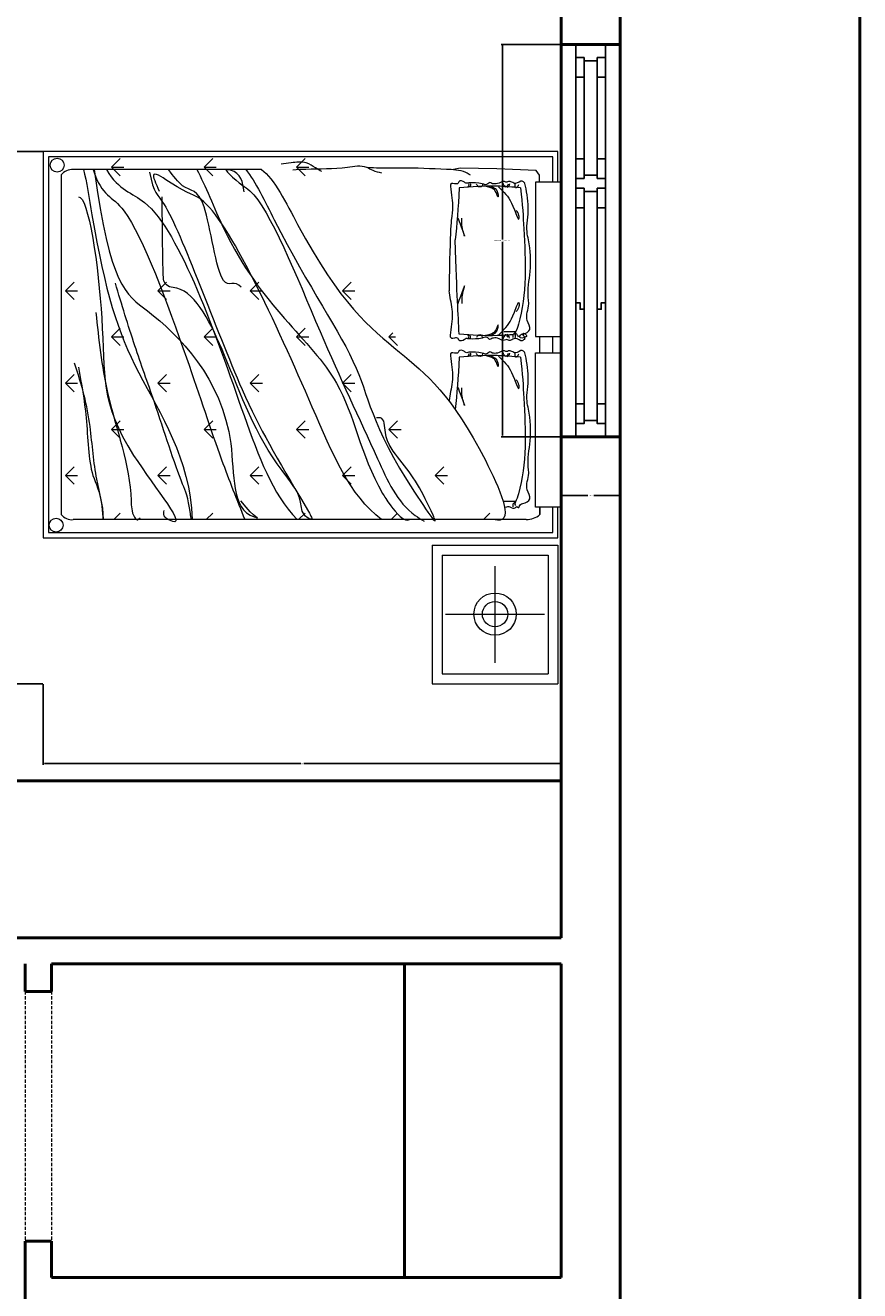
# Model space of a CAD drawing. Units: inches. Extents: x 64 to 1167, y 117 to 939.
# Tile 19 of 56: x 385 to 513, y 583 to 777. Entities that reach past the tile are written whole.
import ezdxf

# ---------------------------------------------------------------- set-up
doc = ezdxf.new("R2010")
doc.units = ezdxf.units.IN
doc.header["$MEASUREMENT"] = 0
doc.linetypes.add('DASHED', pattern=[0.75, 0.5, -0.25])
for name, color, linetype, lineweight in [('A-ANNO-DIMS', 2, 'Continuous', 18), ('A-ANNO-TTLB', 7, 'Continuous', 50), ('A-FLOR-OVHD', 8, 'DASHED', 18), ('A-FURN', 8, 'Continuous', 18), ('A-GLAZ', 4, 'Continuous', 25), ('A-WALL', 7, 'Continuous', 50)]:
    doc.layers.add(name, color=color, linetype=linetype, lineweight=lineweight)
doc.styles.get("Standard").update_dxf_attribs({"font": 'arial.ttf'})
doc.dimstyles.get("Standard").update_dxf_attribs({"dimtxt": 0.18, "dimasz": 0.18, "dimexe": 0.18, "dimexo": 0.0625, "dimgap": 0.09, "dimtad": 0, "dimtih": 1, "dimtoh": 1, "dimdec": 4, "dimzin": 0, "dimdsep": 46, "dimtxsty": 'Standard', "dimcen": 0.09, "dimadec": 0, "dimazin": 0, "dimtfac": 1, "dimtdec": 4, "dimtofl": 0, "dimtmove": 0, "dimatfit": 3, "dimfxl": 1, "dimtolj": 1, "dimtzin": 0, "dimarcsym": 0})

# ---------------------------------------------------------------- blocks, each defined once
blk = doc.blocks.new("W-5'")
for p, q in [((0, 9), (0, 0)), ((0, 9), (60, 9)), ((60, 9), (60, 0)), ((0, 6.75), (60, 6.75)), ((2.000000000000568, 5.5), (20.5, 5.5)), ((57.99999999999977, 5.5), (22.00000000000045, 5.5)), ((0, 2.25), (60, 2.25)), ((2.000000000000568, 3.499999999999886), (20.49999999999966, 3.499999999999886)), ((57.99999999999943, 3.499999999999886), (22.0000000000008, 3.499999999999886)), ((0, 0), (60, 0))]:
    blk.add_line(p, q)
for points in [[(0, 2.25), (0, 6.75), (2, 6.75), (2.000000000000227, 5.5), (2.500000000000227, 5.5), (2.500000000000341, 3.499999999999772), (2.000000000000568, 3.499999999999886), (2.000000000000454, 2.25), (0, 2.25)], [(5.000000000000227, 6.75), (5.000000000000341, 5.49999999999909)], [(17.5, 6.75), (17.49999999999988, 5.49999999999909)], [(25.00000000000046, 6.75), (25.00000000000057, 5.49999999999909)], [(39.50000000000012, 6.75), (39.50000000000023, 6.125), (40.50000000000011, 6.124999999999886), (40.50000000000011, 5.499999999999772)], [(54.99999999999977, 6.75), (54.99999999999966, 5.49999999999909)], [(60, 2.25), (60, 6.75), (58, 6.75), (57.99999999999977, 5.5), (57.49999999999977, 5.5), (57.49999999999966, 3.499999999999772), (57.99999999999943, 3.499999999999886), (57.99999999999954, 2.25), (60, 2.25)], [(5.000000000000341, 3.499999999999772), (5.000000000000454, 2.25)], [(17.49999999999988, 3.499999999999772), (17.49999999999977, 2.25)], [(25.00000000000057, 3.499999999999772), (25.00000000000068, 2.25)], [(39.50000000000012, 2.249999999999772), (39.50000000000023, 2.874999999999772), (40.50000000000011, 2.874999999999886), (40.50000000000011, 3.5)], [(54.99999999999966, 3.499999999999772), (54.99999999999954, 2.25)]]:
    blk.add_lwpolyline(points)
blk.add_lwpolyline([(22.00000000000023, 6.749999999999772), (20.50000000000023, 6.75), (20.5, 5.5), (20, 5.5), (19.99999999999988, 3.499999999999772), (20.49999999999966, 3.499999999999886), (20.49999999999977, 2.25), (22.00000000000023, 2.25), (22.00000000000034, 3.499999999999886), (22.50000000000011, 3.499999999999772), (22.5, 5.5), (22, 5.5)], close=True)
blk = doc.blocks.new('A$C4D3620D9')
for p, q in [((-1.9172435e-09, 0.0787401612884481), (-1.9172435e-09, 3.8081331e-09)), ((0.00467356541461, 0.0787401612884481), (-1.9172435e-09, 0.0787401612884481)), ((0.0007873996574336, 0.0779527597137709), (0.0007873996574336, 0.0007874053830967)), ((0.00467356541461, 0.0779527597137709), (0.0007873996574336, 0.0779527597137709)), ((0.00467356541461, 0.0792544463673569), (0.00467356541461, 0.075317438493112)), ((0.0282956126589336, 0.0792544463673569), (0.00467356541461, 0.0792544463673569)), ((0.0282956126589336, 0.075317438493112), (0.0282956126589336, 0.0792544463673569)), ((0.0307595016168156, 0.0779527597137709), (0.0282956126589336, 0.0779527597137709)), ((0.0307595016168156, 0.0792544463673569), (0.0543815488608528, 0.0792544463673569)), ((0.0307595016168156, 0.075317438493112), (0.0307595016168156, 0.0792544463673569)), ((0.0543815488608528, 0.0792544463673569), (0.0543815488608528, 0.075317438493112)), ((0.0590551161929928, 0.0787401612884481), (0.0543815488608528, 0.0787401612884481)), ((0.0582677146183157, 0.0779527597137709), (0.0543815488608528, 0.0779527597137709)), ((0.0582677146183157, 0.0007874053830967), (0.0582677146183157, 0.0779527597137709)), ((0.0590551161929928, 3.8081331e-09), (0.0590551161929928, 0.0787401612884481)), ((0.0601987849213903, 0.0787401612881616), (0.081403509331693, 0.0787401612881616)), ((0.0601987849222496, 0.0595118148313899), (0.0601987849213903, 0.0787401612881616)), ((0.0814035093314065, 0.0595118148313899), (0.081403509331693, 0.0787401612881616)), ((0.0035794720309878, 0.0759111718182644), (0.0029072656060613, 0.0754310234897705)), ((0.0046357966132882, 0.0759111718182644), (0.0035794720309878, 0.0759111718182644)), ((0.0307595016168156, 0.0759842557766485), (0.0282956126589336, 0.0759842557766485)), ((0.054377727552549, 0.0759842557766485), (0.0555118091065161, 0.0759842557766485)), ((0.0555118091065161, 0.0759842557766485), (0.0543815488608528, 0.0759842557766485)), ((0.0617105959454922, 0.0772283502646326), (0.079891698307591, 0.0772283502646326)), ((0.0617105959457786, 0.0610236258549189), (0.0617105959457786, 0.0772283502646326)), ((0.0708011471263984, 0.0766850431779937), (0.0708011471263984, 0.0615669329415578)), ((0.079891698307591, 0.0610236258549189), (0.079891698307591, 0.0772283502646326)), ((0.0029072656060613, 0.0754310234897705), (0.0026355774045485, 0.0693811549967009)), ((0.00467356541461, 0.075317438493112), (0.0282956126589336, 0.075317438493112)), ((0.0543815488608528, 0.075317438493112), (0.0307595016168156, 0.075317438493112)), ((0.0562992106811932, 0.0738965977054579), (0.0562992106811932, 0.0045665911628336)), ((0.0026355774045485, 0.0693811549967009), (0.0025231474489739, 0.0638114348318388)), ((0.0562992106811932, 0.0673533970283048), (0.0553044557509422, 0.0683481519585558)), ((0.0782090211420629, 0.0691259880597757), (0.0633932731107339, 0.0691259880597757)), ((0.0025231474489739, 0.0638114348318388), (0.0027152066677373, 0.0627551085436987)), ((0.0495592131537562, 0.0599512589318993), (0.048233387939021, 0.0612770841466346)), ((0.0495590589220744, 0.0599512300134053), (0.0495590589220744, 0.0618262300136619)), ((0.0495592131537562, 0.0599512589318993), (0.0508850383684915, 0.0612770841466346)), ((0.0617105959454922, 0.0610236258549189), (0.079891698307591, 0.0610236258549189)), ((0.0601987849222496, 0.0595118148313899), (0.0814035093314065, 0.0595118148313899)), ((0.028346009718279, 0.0528801911199781), (0.0296718349330142, 0.0542060163347133)), ((0.042488145341835, 0.0528801911199781), (0.0411623201270998, 0.0542060163347133)), ((0.0424879959300454, 0.0528801670213763), (0.0424879959300454, 0.0547551670213465)), ((0.042488145341835, 0.0528801911199781), (0.0438139705565702, 0.0542060163347133)), ((0.0562992106811932, 0.0532112614044624), (0.0553044557509422, 0.0542060163347133)), ((0.028346009718279, 0.0528801911199781), (0.0277335089951635, 0.0534926918430935)), ((0.0283458699457009, 0.0528801670213763), (0.0283458699457009, 0.0538887130254105)), ((0.0212749419063577, 0.0458091233083433), (0.0199491166916225, 0.0471349485230785)), ((0.0212748069536719, 0.0458091040293473), (0.0212748069536719, 0.0476841040293175)), ((0.0212749419063577, 0.0458091233083433), (0.022600767121093, 0.0471349485230785)), ((0.0354170775302002, 0.0458091233083433), (0.034091252315465, 0.0471349485230785)), ((0.0354169329380164, 0.0458091040293473), (0.0354169329380164, 0.0476841040293175)), ((0.0354170775302002, 0.0458091233083433), (0.036742902744649, 0.0471349485230785)), ((0.0495592131537562, 0.0458091233083433), (0.048233387939021, 0.0471349485230785)), ((0.0495590589220744, 0.0458091040293473), (0.0495590589220744, 0.0476841040293175)), ((0.0495592131537562, 0.0458091233083433), (0.0508850383684915, 0.0471349485230785)), ((0.0023928504725611, 0.0387380554964221), (0.0010670252578259, 0.0400638807111573)), ((0.0023927203394811, 0.0387380410370318), (0.0023927203394811, 0.040613041037002)), ((0.0023928504725611, 0.0387380554964221), (0.0037186756870099, 0.0400638807111573)), ((0.028346009718279, 0.0387380554964221), (0.0270201845035437, 0.0400638807111573)), ((0.0283458699457009, 0.0387380410370318), (0.0283458699457009, 0.040613041037002)), ((0.028346009718279, 0.0387380554964221), (0.0296718349330142, 0.0400638807111573)), ((0.042488145341835, 0.0387380554964221), (0.0411623201270998, 0.0400638807111573)), ((0.0424879959300454, 0.0387380410370318), (0.0424879959300454, 0.040613041037002)), ((0.042488145341835, 0.0387380554964221), (0.0438139705565702, 0.0400638807111573)), ((0.0562992106811932, 0.0390691257809063), (0.0553044557509422, 0.0400638807111573)), ((0.0027559035945561, 0.0333881572410386), (0.0027559035945561, 0.0045665911628336)), ((0.0212749419063577, 0.0316669876845008), (0.0199491166916225, 0.0329928128992361)), ((0.0212748069536719, 0.0316669780450028), (0.0212748069536719, 0.033541978044973)), ((0.0212749419063577, 0.0316669876845008), (0.022600767121093, 0.0329928128992361)), ((0.0354170775302002, 0.0316669876845008), (0.034091252315465, 0.0329928128992361)), ((0.0354169329380164, 0.0316669780450028), (0.0354169329380164, 0.033541978044973)), ((0.0354170775302002, 0.0316669876845008), (0.036742902744649, 0.0329928128992361)), ((0.0495592131537562, 0.0316669876845008), (0.048233387939021, 0.0329928128992361)), ((0.0495590589220744, 0.0316669780450028), (0.0495590589220744, 0.033541978044973)), ((0.0495592131537562, 0.0316669876845008), (0.0508850383684915, 0.0329928128992361)), ((0.0023928504725611, 0.0245959198725796), (0.0010670252578259, 0.0259217450873148)), ((0.0023927203394811, 0.0245959150529738), (0.0023927203394811, 0.026470915052944)), ((0.0023928504725611, 0.0245959198725796), (0.0037186756870099, 0.0259217450873148)), ((0.028346009718279, 0.0245959198725796), (0.0270201845035437, 0.0259217450873148)), ((0.0283458699457009, 0.0245959150529738), (0.0283458699457009, 0.026470915052944)), ((0.028346009718279, 0.0245959198725796), (0.0296718349330142, 0.0259217450873148)), ((0.042488145341835, 0.0245959198725796), (0.0411623201270998, 0.0259217450873148)), ((0.0424879959300454, 0.0245959150529738), (0.0424879959300454, 0.026470915052944)), ((0.042488145341835, 0.0245959198725796), (0.0438139705565702, 0.0259217450873148)), ((0.0562992106811932, 0.0249269901570639), (0.0553044557509422, 0.0259217450873148)), ((0.0212748069536719, 0.0175248520606583), (0.0212748069536719, 0.0193998520606286)), ((0.0354169329380164, 0.0175248520606583), (0.0354169329380164, 0.0193998520606286)), ((0.0495590589220744, 0.0175248520606583), (0.0495590589220744, 0.0193998520606286)), ((0.0212749419063577, 0.0175248520606583), (0.0199491166916225, 0.0188506772753936)), ((0.0212749419063577, 0.0175248520606583), (0.022600767121093, 0.0188506772753936)), ((0.0354170775302002, 0.0175248520606583), (0.034091252315465, 0.0188506772753936)), ((0.0354170775302002, 0.0175248520606583), (0.036742902744649, 0.0188506772753936)), ((0.0495592131537562, 0.0175248520606583), (0.048233387939021, 0.0188506772753936)), ((0.0495592131537562, 0.0175248520606583), (0.0508850383684915, 0.0188506772753936)), ((0.0023928504725611, 0.0104537842490236), (0.0010670252578259, 0.0117796094637588)), ((0.0023927203394811, 0.0104537890686293), (0.0023927203394811, 0.0123287890685996)), ((0.0023928504725611, 0.0104537842490236), (0.0037186756870099, 0.0117796094637588)), ((0.028346009718279, 0.0104537842490236), (0.0270201845035437, 0.0117796094637588)), ((0.0283458699457009, 0.0104537890686293), (0.0283458699457009, 0.0123287890685996)), ((0.028346009718279, 0.0104537842490236), (0.0296718349330142, 0.0117796094637588)), ((0.042488145341835, 0.0104537842490236), (0.0411623201270998, 0.0117796094637588)), ((0.0424879959300454, 0.0104537890686293), (0.0424879959300454, 0.0123287890685996)), ((0.042488145341835, 0.0104537842490236), (0.0438139705565702, 0.0117796094637588)), ((0.0562992106811932, 0.0107848545335078), (0.0553044557509422, 0.0117796094637588)), ((0.0212749419063577, 0.0033827164371023), (0.0199491166916225, 0.0047085416518375)), ((0.0212748069536719, 0.0033827260766003), (0.0212748069536719, 0.0052577260765705)), ((0.0212749419063577, 0.0033827164371023), (0.022600767121093, 0.0047085416518375)), ((0.0354170775302002, 0.0033827164371023), (0.034091252315465, 0.0047085416518375)), ((0.0354169329380164, 0.0033827260766003), (0.0354169329380164, 0.0052577260765705)), ((0.0354170775302002, 0.0033827164371023), (0.036742902744649, 0.0047085416518375)), ((0.0495592131537562, 0.0033827164371023), (0.048233387939021, 0.0047085416518375)), ((0.0495590589220744, 0.0033827260766003), (0.0495590589220744, 0.0052577260765705)), ((0.0495592131537562, 0.0033827164371023), (0.0508850383684915, 0.0047085416518375)), ((0.0035433051692332, 0.0027559093199327), (0.0555118091065161, 0.0027559093199327)), ((-1.9172435e-09, 3.8081331e-09), (0.0590551161929928, 3.8081331e-09)), ((0.0007873996574336, 0.0007874053830967), (0.0582677146183157, 0.0007874053830967))]:
    blk.add_line(p, q)
for centre, radius in [((0.0707513535392744, 0.0691259880597757), 0.0032325956113447), ((0.0707513535392744, 0.0691259880597757), 0.0019395573668068), ((0.0020742829779404, 0.0021314214566479), 0.001060751545716), ((0.0571487571348163, 0.0019636278839458), 0.001060751545716)]:
    blk.add_circle(centre, radius)
for centre, radius, start, end in [((0.0530791022767488, 0.0738743911488128), 0.0032201849741766, 0.3951177370100151, 40.93480323431428), ((0.0047875531246371, 0.0043735362925772), 0.0020408013122606, 174.5718411969451, 232.4331988533713), ((0.0542675611511121, 0.0043735362925772), 0.0020408013122606, 307.5668011466286, 5.428158803054822)]:
    blk.add_arc(centre, radius, start, end)
for points, knots in [([(0.0048365976513518, 0.0736594542284752), (0.0046865572771571, 0.0735405990503285), (0.0042154124472061, 0.0731673794894229), (0.0051147198561427, 0.0723894111691574), (0.0046436937171123, 0.0717343409572876), (0.0044861351354456, 0.0712431238178855), (0.0047670137325089, 0.0708969222379649), (0.0043951144557003, 0.070429531409413), (0.0049397934298764, 0.0696815480031238), (0.0049695794529733, 0.0691292615394602), (0.0048891960267517, 0.0685844033621719), (0.0046080990017169, 0.0683051057608031), (0.0052360238918854, 0.067836924870102), (0.0047055913065973, 0.0670462991742328), (0.0047897540872062, 0.0654633327115256), (0.0047793161869003, 0.065025374593303), (0.004898831881349, 0.0646567040834141), (0.0044927693017498, 0.0643521638246923), (0.0043384200951436, 0.0636018684404759), (0.0049757629367234, 0.0634671701522252), (0.0049283856853836, 0.0629564768603914), (0.0047328977102659, 0.0621292145196789), (0.0068742889888249, 0.0625949138095424), (0.00945315625115, 0.0626991092817268), (0.0112451995730627, 0.0621988917383554), (0.0212728950173473, 0.0621107047960308)], [0, 0, 0, 0, 13.86455467720318, 43.53637000076386, 61.14632977951814, 74.70103136527402, 82.54942496484034, 92.69911054008931, 117.9632291581877, 145.403589760466, 151.672149812357, 161.8218382801924, 170.6869188427139, 200.2152131796471, 252.8134028960791, 263.1188392314721, 271.6169301537087, 278.2156374531289, 303.0344424988025, 309.9475444343205, 324.5216492986515, 336.9310539839077, 372.0300868404458, 441.1072365570267, 515.2850541027483, 515.2850541027483, 515.2850541027483, 515.2850541027483]), ([(0.0286032373355917, 0.0736594542284752), (0.0283901387790432, 0.0737681360687285), (0.0283107456120852, 0.0734464415634605), (0.0274732602962662, 0.073231979190245), (0.0282668620300998, 0.074214931891628), (0.028770105723018, 0.0727855605982482), (0.0279550156024982, 0.0728974986145838), (0.027894825694588, 0.0736740510074301), (0.0272522530020957, 0.0749265791887947), (0.0254337792797541, 0.0735158175328567), (0.0238547160798468, 0.0744277498250901), (0.0213522999355497, 0.0739966961268728), (0.0181040516137842, 0.0747362754916003), (0.0146729423881414, 0.0745377535684842), (0.0115416732517151, 0.0737807307327391), (0.0088971167878206, 0.0745138215331002), (0.0058949003327802, 0.0739287448956794), (0.0048740866915305, 0.0736969433187834)], [1218.16176084401, 1218.16176084401, 1218.16176084401, 1218.16176084401, 1236.41772560291, 1259.461407570304, 1267.510214435793, 1274.94157530681, 1291.235898423827, 1302.335205769575, 1338.06404694822, 1376.85685403828, 1447.206053446744, 1470.997990578017, 1583.629338998909, 1716.764992750132, 1751.330460865135, 1847.37023741712, 1932.774851490887, 1932.774851490887, 1932.774851490887, 1932.774851490887]), ([(0.005544089258687, 0.0730395393798886), (0.0081682493614572, 0.073330616083179), (0.0147634871443482, 0.073695728793595), (0.0224653586486765, 0.0740458145243227), (0.0272988543415916, 0.0724320017937094), (0.0277439214533936, 0.0722255906952714)], [2.97425896690972, 2.97425896690972, 2.97425896690972, 2.97425896690972, 152.5529234775361, 555.0235128103611, 595.395635729665, 595.395635729665, 595.395635729665, 595.395635729665]), ([(0.0286032373355917, 0.0736594542284752), (0.0287532777100729, 0.0735405990503285), (0.0292244225397374, 0.0731673794894229), (0.0283251151310873, 0.0723894111691574), (0.0287961412698313, 0.0717343409572876), (0.0289536998517844, 0.0712431238178855), (0.0286728212547211, 0.0708969222379649), (0.0290447205315297, 0.070429531409413), (0.0285000415573536, 0.0696815480031238), (0.0284702555342567, 0.0691292615394602), (0.0285506389601918, 0.0685844033621719), (0.0288317359855131, 0.0683051057608031), (0.0282038110953446, 0.067836924870102), (0.0287342436803463, 0.0670462991742328), (0.0286500808997373, 0.0654633327115256), (0.0286605188000432, 0.065025374593303), (0.028541003105881, 0.0646567040834141), (0.0289470656851937, 0.0643521638246923), (0.0291014148918, 0.0636018684404759), (0.0284640720505066, 0.0634671701522252), (0.0285114493015599, 0.0629564768603914), (0.0287069372766776, 0.0621292145196789), (0.0265655459981186, 0.0625949138095424), (0.0239866787357935, 0.0626991092817268), (0.0221946354138809, 0.0621988917383554), (0.0212728950173473, 0.0621107047960308)], [0, 0, 0, 0, 13.86455467720318, 43.53637000076386, 61.14632977951814, 74.70103136527402, 82.54942496484034, 92.69911054008931, 117.9632291581877, 145.403589760466, 151.672149812357, 161.8218382801924, 170.6869188427139, 200.2152131796471, 252.8134028960791, 263.1188392314721, 271.6169301537087, 278.2156374531289, 303.0344424988025, 309.9475444343205, 324.5216492986515, 336.9310539839077, 372.0300868404458, 441.1072365570267, 515.2850541027483, 515.2850541027483, 515.2850541027483, 515.2850541027483]), ([(0.0307502809126048, 0.0736594542284752), (0.0306002405384101, 0.0735405990503285), (0.0301290957084591, 0.0731673794894229), (0.0310284031173957, 0.0723894111691574), (0.0305573769783653, 0.0717343409572876), (0.0303998183966986, 0.0712431238178855), (0.0306806969937619, 0.0708969222379649), (0.0303087977166668, 0.070429531409413), (0.030853476690843, 0.0696815480031238), (0.0308832627139398, 0.0691292615394602), (0.0308028792880048, 0.0685844033621719), (0.0305217822629699, 0.0683051057608031), (0.0311497071531384, 0.067836924870102), (0.0306192745678503, 0.0670462991742328), (0.0307034373484592, 0.0654633327115256), (0.0306929994481533, 0.065025374593303), (0.030812515142602, 0.0646567040834141), (0.0304064525630028, 0.0643521638246923), (0.0302521033563966, 0.0636018684404759), (0.0308894461979764, 0.0634671701522252), (0.0308420689466366, 0.0629564768603914), (0.030646580971519, 0.0621292145196789), (0.0327879722500779, 0.0625949138095424), (0.035366839512403, 0.0626991092817268), (0.0371588828343157, 0.0621988917383554), (0.0380806232308492, 0.0621107047960308)], [0, 0, 0, 0, 13.86455467720318, 43.53637000076386, 61.14632977951814, 74.70103136527402, 82.54942496484034, 92.69911054008931, 117.9632291581877, 145.403589760466, 151.672149812357, 161.8218382801924, 170.6869188427139, 200.2152131796471, 252.8134028960791, 263.1188392314721, 271.6169301537087, 278.2156374531289, 303.0344424988025, 309.9475444343205, 324.5216492986515, 336.9310539839077, 372.0300868404458, 441.1072365570267, 515.2850541027483, 515.2850541027483, 515.2850541027483, 515.2850541027483]), ([(0.0543829123142948, 0.0707506158359475), (0.0543038220402962, 0.0709544075208952), (0.0542244288733382, 0.0714271170690204), (0.0547776091064686, 0.0721016006535524), (0.0541805452913528, 0.072421652131004), (0.054683788984271, 0.0727855605982482), (0.0538686988637512, 0.0728974986145838), (0.053808508955841, 0.0736740510074301), (0.0531659362633487, 0.0749265791887947), (0.0513474625410071, 0.0735158175328567), (0.0497683993410998, 0.0744277498250901), (0.0472659831968027, 0.0739966961268728), (0.0440177348750372, 0.0747362754916003), (0.0405866256493944, 0.0745377535684842), (0.0374553565129681, 0.0737807307327391), (0.0348108000490736, 0.0745138215331002), (0.0318085835940332, 0.0739287448956794), (0.0307877699527835, 0.0736969433187834)], [1218.16176084401, 1218.16176084401, 1218.16176084401, 1218.16176084401, 1236.41772560291, 1259.461407570304, 1267.510214435793, 1274.94157530681, 1291.235898423827, 1302.335205769575, 1338.06404694822, 1376.85685403828, 1447.206053446744, 1470.997990578017, 1583.629338998909, 1716.764992750132, 1751.330460865135, 1847.37023741712, 1932.774851490887, 1932.774851490887, 1932.774851490887, 1932.774851490887]), ([(0.0314577725196535, 0.0730395393798886), (0.0340819326224237, 0.073330616083179), (0.0406771704056012, 0.073695728793595), (0.0483790419099295, 0.0740458145243227), (0.0532125376028446, 0.0724320017937094), (0.0536576047146466, 0.0722255906952714)], [2.97425896690972, 2.97425896690972, 2.97425896690972, 2.97425896690972, 152.5529234775361, 555.0235128103611, 595.395635729665, 595.395635729665, 595.395635729665, 595.395635729665]), ([(0.0027559035945561, 0.0333881572410386), (0.004068861814208, 0.0353052018069471), (0.0224327175217652, 0.0442945305349701), (0.0302023836597732, 0.0540227246775309), (0.0386310718371762, 0.0642063363210489), (0.0571141568291314, 0.0722848152248285), (0.0562744531497464, 0.0690659459354448), (0.0562744531497464, 0.0690659459354448)], [63.61308249396958, 63.61308249396958, 63.61308249396958, 63.61308249396958, 240.8947408841979, 911.6915771060609, 1510.287228053419, 1760.643600742247, 1779.956830290146, 1779.956830290146, 1779.956830290146, 1779.956830290146]), ([(0.0050615318915642, 0.072722226496686), (0.0051476382388615, 0.0726975445784803), (0.0053560412068935, 0.0726378069965166), (0.0057170899813137, 0.0721954282224348), (0.0052227720321595, 0.0721975850136392), (0.0050450293407968, 0.0721974298166039), (0.0049865538114934, 0.0721973787582875)], [0, 0, 0, 0, 7.251906870029622, 17.55177136899566, 27.26256586803696, 32.02367395246505, 32.02367395246505, 32.02367395246505, 32.02367395246505]), ([(0.005544089258687, 0.0730395393798886), (0.0054285326611327, 0.0718430517612948), (0.0051465754371547, 0.0687041249782522), (0.0053778859187082, 0.0655581503655069), (0.005538618127567, 0.0636112192442515)], [12.00866106341675, 12.00866106341675, 12.00866106341675, 12.00866106341675, 110.9809201442566, 271.6334972433642, 271.6334972433642, 271.6334972433642, 271.6334972433642]), ([(0.0053767616179722, 0.0696538298154881), (0.0055842022151424, 0.0698629121603073), (0.006622707500298, 0.0709096364892138), (0.0075337771401011, 0.0716639264812945), (0.0108873150249536, 0.0727992150415786), (0.0095654697358305, 0.0728301700544003), (0.0092114712549126, 0.0725361731856251), (0.0089878138908351, 0.0723504250308047)], [0, 0, 0, 0, 21.82548878043965, 109.2644628480433, 148.7034500082113, 161.9316867812909, 184.6305298977724, 184.6305298977724, 184.6305298977724, 184.6305298977724]), ([(0.0280630733692578, 0.0696538298154881), (0.0278556327718011, 0.0698629121603073), (0.0268171274866455, 0.0709096364892138), (0.0259060578471289, 0.0716639264812945), (0.0225525199619899, 0.0727992150415786), (0.0238743652511131, 0.0728301700544003), (0.0242283637320309, 0.0725361731856251), (0.0244520210961084, 0.0723504250308047)], [0, 0, 0, 0, 21.82548878043965, 109.2644628480433, 148.7034500082113, 161.9316867812909, 184.6305298977724, 184.6305298977724, 184.6305298977724, 184.6305298977724]), ([(0.0282009882337618, 0.0722899867354514), (0.0281211918194831, 0.0722251085407631), (0.027961598924468, 0.0720953520975332), (0.0275311046648921, 0.072435523068448), (0.0279488048794534, 0.0717835391012381), (0.0282527695234185, 0.0718195843677047), (0.0284259224739742, 0.0718401174936292)], [0, 0, 0, 0, 7.251905290411031, 14.5038166296127, 24.80368477899669, 38.43742430517991, 38.43742430517991, 38.43742430517991, 38.43742430517991]), ([(0.0283783030953794, 0.072722226496686), (0.0282921967483685, 0.0726975445784803), (0.0280837937800501, 0.0726378069965166), (0.0277227450056299, 0.0721954282224348), (0.0282170629550705, 0.0721975850136392), (0.0283948056461467, 0.0721974298166039), (0.0284532811754502, 0.0721973787582875)], [0, 0, 0, 0, 7.251906870029622, 17.55177136899566, 27.26256586803696, 32.02367395246505, 32.02367395246505, 32.02367395246505, 32.02367395246505]), ([(0.0280027437280139, 0.07188249190508), (0.0280113023260973, 0.0718430517612948), (0.0282932595497888, 0.0687041249782522), (0.0280619490682354, 0.0655581503655069), (0.0279012168593765, 0.0636112192442515)], [12.00866106341675, 12.00866106341675, 12.00866106341675, 12.00866106341675, 110.9809201442566, 271.6334972433642, 271.6334972433642, 271.6334972433642, 271.6334972433642]), ([(0.0309752151528172, 0.072722226496686), (0.0310613214998281, 0.0726975445784803), (0.0312697244681465, 0.0726378069965166), (0.0316307732425667, 0.0721954282224348), (0.0311364552934125, 0.0721975850136392), (0.0309587126020498, 0.0721974298166039), (0.0309002370727464, 0.0721973787582875)], [0, 0, 0, 0, 7.251906870029622, 17.55177136899566, 27.26256586803696, 32.02367395246505, 32.02367395246505, 32.02367395246505, 32.02367395246505]), ([(0.0314577725196535, 0.0730395393798886), (0.0313422159223857, 0.0718430517612948), (0.0310602586984077, 0.0687041249782522), (0.0312915691799612, 0.0655581503655069), (0.03145230138882, 0.0636112192442515)], [12.00866106341675, 12.00866106341675, 12.00866106341675, 12.00866106341675, 110.9809201442566, 271.6334972433642, 271.6334972433642, 271.6334972433642, 271.6334972433642]), ([(0.0312904448789388, 0.0696538298154881), (0.0314978854763954, 0.0698629121603073), (0.032536390761551, 0.0709096364892138), (0.0334474604010676, 0.0716639264812945), (0.0368009982862066, 0.0727992150415786), (0.0354791529970835, 0.0728301700544003), (0.0351251545161656, 0.0725361731856251), (0.0349014971520881, 0.0723504250308047)], [0, 0, 0, 0, 21.82548878043965, 109.2644628480433, 148.7034500082113, 161.9316867812909, 184.6305298977724, 184.6305298977724, 184.6305298977724, 184.6305298977724]), ([(0.0541146714950148, 0.0722899867354514), (0.0540348750807361, 0.0722251085407631), (0.053875282185721, 0.0720953520975332), (0.0534447879261451, 0.072435523068448), (0.0538624881407064, 0.0717835391012381), (0.0541664527846715, 0.0718195843677047), (0.0543396057349407, 0.0718401174936292)], [0, 0, 0, 0, 7.251905290411031, 14.5038166296127, 24.80368477899669, 38.43742430517991, 38.43742430517991, 38.43742430517991, 38.43742430517991]), ([(0.0049865538114934, 0.0711476835974503), (0.0050687765542534, 0.0710995338273264), (0.0052163014454239, 0.0710131430135757), (0.0055438346270972, 0.0708411199098117), (0.0051897840703747, 0.0704474317378091), (0.0049226502086976, 0.0703697502779785), (0.0047616193123257, 0.0703229231365858)], [0, 0, 0, 0, 7.677058644127298, 13.77425765586811, 22.75751049019892, 36.39126008106757, 36.39126008106757, 36.39126008106757, 36.39126008106757]), ([(0.0049115757314226, 0.0713351292071147), (0.0050483925622571, 0.0713155846704209), (0.00528756023958, 0.0712814191264063), (0.0054180631402025, 0.0710827478224377), (0.0054739113320967, 0.0709977272362173)], [0, 0, 0, 0, 9.941487798237118, 17.37858226137827, 17.37858226137827, 17.37858226137827, 17.37858226137827]), ([(0.0285282592555209, 0.0713351292071147), (0.0283914424249729, 0.0713155846704209), (0.0281522747473636, 0.0712814191264063), (0.0280217718470275, 0.0710827478224377), (0.0279659236551333, 0.0709977272362173)], [0, 0, 0, 0, 9.941487798237118, 17.37858226137827, 17.37858226137827, 17.37858226137827, 17.37858226137827]), ([(0.0284532811754502, 0.0711476835974503), (0.0283710584329766, 0.0710995338273264), (0.0282235335418061, 0.0710131430135757), (0.0278960003598463, 0.0708411199098117), (0.0282500509168553, 0.0704474317378091), (0.0285171847782459, 0.0703697502779785), (0.0286782156749043, 0.0703229231365858)], [0, 0, 0, 0, 7.677058644127298, 13.77425765586811, 22.75751049019892, 36.39126008106757, 36.39126008106757, 36.39126008106757, 36.39126008106757]), ([(0.0309002370727464, 0.0711476835974503), (0.0309824598155064, 0.0710995338273264), (0.0311299847066769, 0.0710131430135757), (0.0314575178883502, 0.0708411199098117), (0.0311034673313412, 0.0704474317378091), (0.0308363334699506, 0.0703697502779785), (0.0306753025735787, 0.0703229231365858)], [0, 0, 0, 0, 7.677058644127298, 13.77425765586811, 22.75751049019892, 36.39126008106757, 36.39126008106757, 36.39126008106757, 36.39126008106757]), ([(0.0308252589926756, 0.0713351292071147), (0.0309620758235101, 0.0713155846704209), (0.031201243500833, 0.0712814191264063), (0.031331746401169, 0.0710827478224377), (0.0313875945933497, 0.0709977272362173)], [0, 0, 0, 0, 9.941487798237118, 17.37858226137827, 17.37858226137827, 17.37858226137827, 17.37858226137827]), ([(0.0052899622935761, 0.068438635749972), (0.0054952627056261, 0.0689413576241006), (0.0057675643053133, 0.0696081462059895), (0.0072006947551368, 0.069606542755945), (0.0062252651550234, 0.0693281447940793), (0.005576434505058, 0.0688895982637219), (0.0053949892610508, 0.0681091758256868), (0.0052899622935761, 0.067657439531032)], [0, 0, 0, 0, 40.53304955345188, 53.76128632653185, 65.633991006901, 89.4815419033458, 122.2568946043973, 122.2568946043973, 122.2568946043973, 122.2568946043973]), ([(0.028149872693654, 0.068438635749972), (0.0279445722816039, 0.0689413576241006), (0.0276722706816302, 0.0696081462059895), (0.0262391402318067, 0.069606542755945), (0.0272145698319201, 0.0693281447940793), (0.027863400482172, 0.0688895982637219), (0.0280448457258928, 0.0681091758256868), (0.028149872693654, 0.067657439531032)], [0, 0, 0, 0, 40.53304955345188, 53.76128632653185, 65.633991006901, 89.4815419033458, 122.2568946043973, 122.2568946043973, 122.2568946043973, 122.2568946043973]), ([(0.0312036455548291, 0.068438635749972), (0.0314089459668791, 0.0689413576241006), (0.0316812475665663, 0.0696081462059895), (0.0331143780163898, 0.069606542755945), (0.0321389484162764, 0.0693281447940793), (0.031490117766311, 0.0688895982637219), (0.0313086725223038, 0.0681091758256868), (0.0312036455548291, 0.067657439531032)], [0, 0, 0, 0, 40.53304955345188, 53.76128632653185, 65.633991006901, 89.4815419033458, 122.2568946043973, 122.2568946043973, 122.2568946043973, 122.2568946043973]), ([(0.005024042851672, 0.0672113265868324), (0.0051598533935062, 0.0671682864776813), (0.0054407661403053, 0.0670792616117291), (0.0054102507302438, 0.066526814729528), (0.0051369276196227, 0.0663637898667114), (0.0049865538114934, 0.0662740986972065)], [0, 0, 0, 0, 9.803724681781771, 20.27818454014789, 33.08902923982005, 33.08902923982005, 33.08902923982005, 33.08902923982005]), ([(0.028415792135558, 0.0672113265868324), (0.0282799815937238, 0.0671682864776813), (0.0279990688466383, 0.0670792616117291), (0.0280295842569862, 0.066526814729528), (0.0283029073673208, 0.0663637898667114), (0.0284532811754502, 0.0662740986972065)], [0, 0, 0, 0, 9.803724681781771, 20.27818454014789, 33.08902923982005, 33.08902923982005, 33.08902923982005, 33.08902923982005]), ([(0.030937726112925, 0.0672113265868324), (0.0310735366547592, 0.0671682864776813), (0.0313544494015583, 0.0670792616117291), (0.0313239339914968, 0.066526814729528), (0.0310506108808758, 0.0663637898667114), (0.0309002370727464, 0.0662740986972065)], [0, 0, 0, 0, 9.803724681781771, 20.27818454014789, 33.08902923982005, 33.08902923982005, 33.08902923982005, 33.08902923982005]), ([(0.0035794720309878, 0.0653479094484727), (0.0034417930584723, 0.0651282414902363), (0.0030224732670215, 0.064459213236538), (0.0027789125091458, 0.0631831200145081), (0.0026375088756734, 0.0598828406738875), (0.002464771656435, 0.0559697489407831), (0.0025745561222319, 0.0519300173558675), (0.0024656294230885, 0.0501996790062119), (0.0024271181197452, 0.049587913610279)], [0, 0, 0, 0, 19.66507286068931, 59.89261910904335, 96.56113180924471, 272.247910760633, 357.6182792033167, 404.3086958409559, 404.3086958409559, 404.3086958409559, 404.3086958409559]), ([(0.0048740866915305, 0.0653368709651308), (0.0050832049317422, 0.06536306439249), (0.0053578763635321, 0.0653974687855683), (0.0053910225662233, 0.0651669515896425), (0.0053989332520259, 0.0651119362654446)], [0, 0, 0, 0, 12.5245209222339, 16.45063618512036, 16.45063618512036, 16.45063618512036, 16.45063618512036]), ([(0.0049490647716012, 0.0650744471751364), (0.0050568069448451, 0.0650932089651694), (0.0052597807488504, 0.0651285540095167), (0.0053800119781582, 0.0649641411159899), (0.0054364222919181, 0.0648870015654719)], [0, 0, 0, 0, 7.617772935087486, 14.35100391219739, 14.35100391219739, 14.35100391219739, 14.35100391219739]), ([(0.0101162066620039, 0.0634100687253293), (0.0104843810756185, 0.0635490454909255), (0.0112207299630033, 0.0638269990444615), (0.013440840744792, 0.064648744938588), (0.0116743539461379, 0.0640159537814059), (0.0108565955956083, 0.0640169052346073), (0.0102030059864, 0.0640176656790257)], [0, 0, 0, 0, 37.67402926178966, 75.348064685456, 89.29184718837381, 144.80492040049, 144.80492040049, 144.80492040049, 144.80492040049]), ([(0.0233236283249397, 0.0634100687253293), (0.0229554539116115, 0.0635490454909255), (0.0222191050239402, 0.0638269990444615), (0.019998994242438, 0.064648744938588), (0.0217654810408057, 0.0640159537814059), (0.0225832393913352, 0.0640169052346073), (0.02323682900083, 0.0640176656790257)], [0, 0, 0, 0, 37.67402926178966, 75.348064685456, 89.29184718837381, 144.80492040049, 144.80492040049, 144.80492040049, 144.80492040049]), ([(0.0284907702156288, 0.0650744471751364), (0.0283830280420985, 0.0650932089651694), (0.0281800542380931, 0.0651285540095167), (0.0280598230090718, 0.0649641411159899), (0.0280034126950255, 0.0648870015654719)], [0, 0, 0, 0, 7.617772935087486, 14.35100391219739, 14.35100391219739, 14.35100391219739, 14.35100391219739]), ([(0.0285657482956995, 0.0653368709651308), (0.0283566300552013, 0.06536306439249), (0.0280819586236979, 0.0653974687855683), (0.0280488124207202, 0.0651669515896425), (0.0280409017352041, 0.0651119362654446)], [0, 0, 0, 0, 12.5245209222339, 16.45063618512036, 16.45063618512036, 16.45063618512036, 16.45063618512036]), ([(0.0307877699527835, 0.0653368709651308), (0.0309968881929952, 0.06536306439249), (0.0312715596247851, 0.0653974687855683), (0.0313047058274763, 0.0651669515896425), (0.0313126165132789, 0.0651119362654446)], [0, 0, 0, 0, 12.5245209222339, 16.45063618512036, 16.45063618512036, 16.45063618512036, 16.45063618512036]), ([(0.0308627480328542, 0.0650744471751364), (0.0309704902060981, 0.0650932089651694), (0.0311734640101034, 0.0651285540095167), (0.0312936952394112, 0.0649641411159899), (0.0313501055531711, 0.0648870015654719)], [0, 0, 0, 0, 7.617772935087486, 14.35100391219739, 14.35100391219739, 14.35100391219739, 14.35100391219739]), ([(0.0360298899232569, 0.0634100687253293), (0.0363980643368715, 0.0635490454909255), (0.0371344132242563, 0.0638269990444615), (0.039354524006045, 0.064648744938588), (0.0375880372073908, 0.0640159537814059), (0.0367702788568613, 0.0640169052346073), (0.036116689247653, 0.0640176656790257)], [0, 0, 0, 0, 37.67402926178966, 75.348064685456, 89.29184718837381, 144.80492040049, 144.80492040049, 144.80492040049, 144.80492040049]), ([(0.0027559035945561, 0.0309899707851193), (0.0045605611227275, 0.0324626402624293), (0.0192588588054884, 0.039441203787317), (0.0334433391173489, 0.0498012866740991), (0.0432506878714203, 0.050384877358165), (0.0573126327109044, 0.0603697703641727), (0.0522039189947793, 0.0581767147360645), (0.0483558930692219, 0.0557996621211614), (0.0442910301834794, 0.0520976029636543), (0.0406017699292641, 0.0522733626188367), (0.0407040258190631, 0.0512126794176687), (0.0407246717229036, 0.0509985229196957)], [77.29953625855738, 77.29953625855738, 77.29953625855738, 77.29953625855738, 271.44428497273, 1004.954987376899, 1678.042926097376, 1756.785404910114, 1778.860099258886, 2050.922655263849, 2181.131765007206, 2245.945302622962, 2262.34199771587, 2262.34199771587, 2262.34199771587, 2262.34199771587]), ([(0.0061289919855387, 0.0307182633492974), (0.0047143706343183, 0.0305201429155276), (0.0030674286081623, 0.0302894855256483), (0.0026818161077388, 0.0277423182121748), (0.0050797207638146, 0.0300698299654718), (0.0061858850106754, 0.0336708416614597), (0.0282319768689555, 0.0423308277742591), (0.0435964615061544, 0.0496871676797292), (0.0541655733909501, 0.05435501430595), (0.056250325594772, 0.0578027746995236), (0.0565301173024121, 0.0582654938496733)], [0, 0, 0, 0, 98.76936717192127, 114.9900795214054, 129.9040091966386, 276.9890476394158, 866.54705065972, 1383.249978258196, 1647.643273655354, 1688.62757872867, 1688.62757872867, 1688.62757872867, 1688.62757872867]), ([(0.0027559035945561, 0.0234944912855693), (0.0050979905048964, 0.0248021711408588), (0.0224288414942498, 0.0312806503414351), (0.0322600560630378, 0.0466415294282543), (0.0466413166231084, 0.0484736261841329), (0.0538155443854786, 0.0528363395206961), (0.0568209644309066, 0.0552600690952111), (0.056239270174204, 0.0561326118651319)], [30.00801097264493, 30.00801097264493, 30.00801097264493, 30.00801097264493, 251.6903052102366, 1114.748003016132, 1738.966639452677, 1789.003382715574, 1846.39181554075, 1846.39181554075, 1846.39181554075, 1846.39181554075]), ([(0.0032913834829957, 0.051807727648152), (0.0031952915490214, 0.0513484190696187), (0.0030254136152679, 0.0505364217564434), (0.001990661585296, 0.0489773801431096), (0.0027566782147743, 0.0453111380949391), (0.0026213803280335, 0.0416364767254096), (0.002774317349469, 0.0388452999130983), (0.0028112359966796, 0.0381715162161061)], [0, 0, 0, 0, 35.51460233006582, 62.78515802390836, 138.3989115663393, 299.5492488157861, 350.8295090751034, 350.8295090751034, 350.8295090751034, 350.8295090751034]), ([(0.0562992106811932, 0.0517632971221204), (0.0524916005182547, 0.0468234103915509), (0.0354954889089426, 0.0398450660511625), (0.0065382040441715, 0.0265643113191005), (0.0066076736279289, 0.0220141290201999), (0.0024208217165703, 0.0160785992545608), (0.0048818954869997, 0.0172181559030396), (0.0060303405905326, 0.0177499230805666)], [72.523447062991, 72.523447062991, 72.523447062991, 72.523447062991, 555.7955723005688, 1402.734709742427, 1609.291454351686, 1686.551304567261, 1754.147494494768, 1754.147494494768, 1754.147494494768, 1754.147494494768]), ([(0.003065054968786, 0.0426222157771044), (0.0028779494823539, 0.0423016358938299), (0.0024213896042028, 0.041519382443301), (0.0014121957872875, 0.0400868788791003), (0.0016972804610484, 0.0381569085177722), (0.0018512029737036, 0.0368874760906191), (0.0019127010575433, 0.0363802880211573)], [0, 0, 0, 0, 28.44515441574033, 69.4095959715559, 128.5182368357245, 167.8484032762137, 167.8484032762137, 167.8484032762137, 167.8484032762137]), ([(0.0031466057433451, 0.0162536663021714), (0.0064185187548851, 0.0168852432844995), (0.0068745975916922, 0.0192531606238143), (0.0378332179712657, 0.0301286465673195), (0.0465106123279896, 0.0355775151438425), (0.056649821778456, 0.0415207844822348), (0.0554771216526191, 0.0394609867342254), (0.0524204305263019, 0.0395583263018598), (0.0450950777166162, 0.0330628554460361), (0.0323171760275842, 0.0285186646355515), (0.020497586593542, 0.0229606893329284), (0.0208018549775139, 0.0186278975570889), (0.0191482925967691, 0.0182776664550197), (0.0069338491551558, 0.0181922205294942)], [0, 0, 0, 0, 256.3585376873524, 961.1430489908762, 1456.615657880957, 1496.398656853854, 1521.751735370274, 1579.397511356921, 1721.860635441086, 2221.555348762143, 2619.707346060348, 2716.49598440807, 2747.72958625681, 2747.72958625681, 2747.72958625681, 2747.72958625681]), ([(0.0027559035945561, 0.0096671632774643), (0.0060163610917906, 0.0116246864751351), (0.0068171149504501, 0.0191866892986238), (0.036143784746805, 0.0290918573445533), (0.0522142105927649, 0.034989959355061), (0.0562992106811932, 0.0388411629511232)], [30.47247939716372, 30.47247939716372, 30.47247939716372, 30.47247939716372, 343.7685381516175, 1242.225509837897, 1706.897848485674, 1706.897848485674, 1706.897848485674, 1706.897848485674]), ([(0.0027559035945561, 0.0078038280718299), (0.020619893373977, 0.0101954558835934), (0.0234621457727951, 0.0160611705462894), (0.0377105401135549, 0.0304805163794686), (0.0548819838559569, 0.0286959922888182), (0.0561423211315634, 0.0332526040188881), (0.0563738264059708, 0.0325773699600048), (0.0534277484947829, 0.0302471792644259)], [14.75935490083986, 14.75935490083986, 14.75935490083986, 14.75935490083986, 546.5438262472209, 1305.510166850577, 1658.181573556414, 1671.144301336132, 1740.950672591642, 1740.950672591642, 1740.950672591642, 1740.950672591642]), ([(0.0027559035945561, 0.0076225406175624), (0.0070375758133289, 0.0090411468895975), (0.0058855675914262, 0.0126228881986673), (0.0312175010391704, 0.0219703917479826), (0.045566320529654, 0.0265719778206145), (0.0532590117133415, 0.0296217546668582), (0.0562992106811932, 0.0308348672126702)], [14.54528061937707, 14.54528061937707, 14.54528061937707, 14.54528061937707, 385.2563712331414, 939.1297608178792, 1351.7431464738, 1621.805854599489, 1621.805854599489, 1621.805854599489, 1621.805854599489]), ([(0.0207426843398863, 0.0302709046207913), (0.0195844685791728, 0.0293183942241425), (0.0225705830357977, 0.0269174975802866), (0.0051797682185787, 0.0248931981283437), (0.0063745822652296, 0.0218780846265099), (0.0037213659860876, 0.0199042871907467), (0.0027559035945561, 0.0191753465100994)], [0, 0, 0, 0, 122.9750891810354, 309.9708726794992, 482.9150002786682, 582.6883579231064, 582.6883579231064, 582.6883579231064, 582.6883579231064]), ([(0.0027559035945561, 0.0061654650344853), (0.0044729340366958, 0.0065987562251623), (0.0203667349359328, 0.0091166764047564), (0.0332323627840447, 0.0131302578745989), (0.0468676201134666, 0.022475063364197), (0.0562992106811932, 0.0227991669069482)], [5.843151847676457, 5.843151847676457, 5.843151847676457, 5.843151847676457, 152.1117047510946, 856.5128561497694, 1549.056257038164, 1549.056257038164, 1549.056257038164, 1549.056257038164]), ([(0.0069338491551558, 0.0053679386098703), (0.0066319188380025, 0.0069245462727276), (0.030328133561136, 0.0102261096674731), (0.0409971127900942, 0.00809437048723), (0.0585744126224235, 0.023117718617897), (0.0558567774199283, 0.0183235992801029), (0.0551832207382563, 0.0184404380715431), (0.0548893558662376, 0.0184914134646762)], [0, 0, 0, 0, 415.3461371885351, 880.9487679787389, 1169.160160302978, 1196.316285765579, 1217.333940450164, 1217.333940450164, 1217.333940450164, 1217.333940450164]), ([(0.0562992106811932, 0.0226417248743778), (0.0559898400333766, 0.0226028820778327), (0.0529490007357085, 0.0222196842508948), (0.0494584602573758, 0.0206079724498916), (0.0393018600129656, 0.0174156167827099), (0.0295189375589592, 0.0138710598774941), (0.0233615739529427, 0.0120075855515398), (0.0201462071431241, 0.0110344818204171)], [1611.74761399537, 1611.74761399537, 1611.74761399537, 1611.74761399537, 1627.688578862765, 1754.960966629267, 2119.233796006786, 2370.723673868909, 2645.581963113626, 2645.581963113626, 2645.581963113626, 2645.581963113626]), ([(0.02461978637708, 0.0080520906652334), (0.0287016972208049, 0.0084855462384124), (0.038374574923089, 0.0095127031047701), (0.0488001858022873, 0.0136226715667148), (0.0552309536143421, 0.0134497866859269), (0.0564888257253274, 0.0143457905368286), (0.0561757781064458, 0.014651211107933), (0.0560177195496173, 0.0148054187484663)], [0, 0, 0, 0, 313.8938139169451, 743.8321388243025, 810.1583525650362, 823.6690259378931, 837.447272684459, 837.447272684459, 837.447272684459, 837.447272684459]), ([(0.0562992106811932, 0.0092384842183513), (0.0538200964666165, 0.0091526021561714), (0.0498054892371393, 0.007851343686389), (0.0430922377557818, 0.0074127960967209), (0.037180504222356, 0.0063548063808698), (0.0340065293328119, 0.0053092460035173), (0.0323739904514674, 0.0047714604105155)], [712.0385222866953, 712.0385222866953, 712.0385222866953, 712.0385222866953, 885.2659301028381, 1108.473028566872, 1241.932247708364, 1383.279253410566, 1383.279253410566, 1383.279253410566, 1383.279253410566]), ([(0.0329704676482297, 0.0053679386098703), (0.0354825467371756, 0.0058378501094334), (0.040831483890693, 0.0068384265207675), (0.0489946996593091, 0.0068612717904767), (0.0520707269113944, 0.0088191889875544), (0.0556459155566298, 0.0091015892225344), (0.0562992106811932, 0.009146614803593)], [0, 0, 0, 0, 215.6645128626575, 459.2116269712382, 591.5328658699049, 630.252873974419, 630.252873974419, 630.252873974419, 630.252873974419])]:
    blk.add_open_spline(points, degree=3, knots=knots)
for points in [[(0.0275916440318903, 0.0722961747142538), (0.0275896346358322, 0.0716901835492206), (0.0275886602934421, 0.0710842047046181), (0.0275910042646716, 0.0704782653578665)], [(0.0535053272931433, 0.0722961747142538), (0.0535033178970852, 0.0716901835492206), (0.0535023435546951, 0.0710842047046181), (0.0535046875259246, 0.0704782653578665)], [(0.005538618127567, 0.0636112192442515), (0.0087301302935555, 0.0634971564334513), (0.0110901816867592, 0.0632889219539677), (0.0135090046009511, 0.0630349601983546)], [(0.0279012168593765, 0.0636112192442515), (0.024709704693388, 0.0634971564334513), (0.0223496533001844, 0.0632889219539677), (0.0135090046009511, 0.0630349601983546)], [(0.03145230138882, 0.0636112192442515), (0.0346438135548085, 0.0634971564334513), (0.0370038649480122, 0.0632889219539677), (0.0394226878622041, 0.0630349601983546)]]:
    blk.add_open_spline(points, degree=3)
blk = doc.blocks.new('*D70')
at = {"layer": 'A-ANNO-DIMS', "color": 0, "lineweight": -2, "transparency": 16777216}
for p, q in [((467.0447888543382, 773.8415699321663), (457.9272888543384, 773.8415699321663)), ((458.1072888543384, 773.6615699321663), (458.1072888543384, 744.024700900788)), ((458.1072888543384, 714.021569932166), (458.1072888543384, 743.658438963544)), ((467.0447888543382, 713.8415699321661), (457.9272888543384, 713.8415699321661))]:
    blk.add_line(p, q, dxfattribs=at)
for points in [[(458.0772888543385, 773.6615699321663), (458.1372888543383, 773.6615699321663), (458.1072888543384, 773.8415699321663)], [(458.0772888543385, 714.021569932166), (458.1372888543383, 714.021569932166), (458.1072888543384, 713.8415699321661)]]:
    blk.add_solid(points, dxfattribs=at)
at = {"layer": 'Defpoints', "color": 0, "lineweight": -2, "transparency": 16777216}
for p in [(467.1072888543382, 773.8415699321663), (458.1072888543384, 713.8415699321661), (467.1072888543382, 713.8415699321661)]:
    blk.add_point(p, dxfattribs=at)
at = {"layer": 'A-ANNO-DIMS', "color": 0, "transparency": 16777216, "insert": (458.1072888543385, 743.8415699321658), "char_height": 0.18, "attachment_point": 5}
blk.add_mtext("\\A1;WINDOW W-5' 60 TYP.", dxfattribs=at)
blk = doc.blocks.new('*D71')
at = {"layer": 'A-ANNO-DIMS', "color": 0, "lineweight": -2, "transparency": 16777216}
for p, q in [((467.1072888543379, 713.7790699321658), (467.1072888543379, 704.6615699321659)), ((476.1072888543379, 713.7790699321658), (476.1072888543379, 704.6615699321659)), ((467.287288854338, 704.8415699321658), (471.1491237793039, 704.8415699321658)), ((475.9272888543379, 704.8415699321658), (472.0654539293721, 704.8415699321658))]:
    blk.add_line(p, q, dxfattribs=at)
for points in [[(467.287288854338, 704.8715699321657), (467.287288854338, 704.8115699321658), (467.1072888543379, 704.8415699321658)], [(475.9272888543379, 704.8715699321657), (475.9272888543379, 704.8115699321658), (476.1072888543379, 704.8415699321658)]]:
    blk.add_solid(points, dxfattribs=at)
at = {"layer": 'Defpoints', "color": 0, "lineweight": -2, "transparency": 16777216}
for p in [(467.1072888543379, 713.8415699321658), (476.1072888543379, 713.8415699321658), (476.1072888543379, 704.8415699321658)]:
    blk.add_point(p, dxfattribs=at)
at = {"layer": 'A-ANNO-DIMS', "color": 0, "transparency": 16777216, "insert": (471.6072888543379, 704.8415699321658), "char_height": 0.18, "attachment_point": 5}
blk.add_mtext('\\A1;9 TYP.', dxfattribs=at)
blk = doc.blocks.new('*D78')
at = {"layer": 'A-ANNO-DIMS', "color": 0, "lineweight": -2, "transparency": 16777216}
for p, q in [((387.7903462954009, 757.4471057688899), (375.4623196080605, 757.4471057688899)), ((375.6423196080604, 757.26710576889), (375.6423196080604, 716.9284811130437)), ((375.6423196080604, 676.2235945199534), (375.6423196080604, 716.5622191757996)), ((387.7903462954009, 676.0435945199534), (375.4623196080605, 676.0435945199534))]:
    blk.add_line(p, q, dxfattribs=at)
for points in [[(375.6123196080605, 757.26710576889), (375.6723196080604, 757.26710576889), (375.6423196080604, 757.4471057688899)], [(375.6123196080605, 676.2235945199534), (375.6723196080604, 676.2235945199534), (375.6423196080604, 676.0435945199534)]]:
    blk.add_solid(points, dxfattribs=at)
at = {"layer": 'Defpoints', "color": 0, "lineweight": -2, "transparency": 16777216}
for p in [(387.8528462954009, 757.4471057688899), (375.6423196080604, 676.0435945199534), (387.8528462954009, 676.0435945199534)]:
    blk.add_point(p, dxfattribs=at)
at = {"layer": 'A-ANNO-DIMS', "color": 0, "transparency": 16777216, "insert": (375.6423196080606, 716.7453501444215), "char_height": 0.18, "attachment_point": 5}
blk.add_mtext('\\A1;DOUBLE BED 81', dxfattribs=at)
blk = doc.blocks.new('*D79')
at = {"layer": 'A-ANNO-DIMS', "color": 0, "lineweight": -2, "transparency": 16777216}
for p, q in [((387.8528462954007, 675.9810945199532), (387.8528462954007, 663.6530678326128)), ((467.1072888546245, 675.9810945199532), (467.1072888546245, 663.6530678326128)), ((388.0328462954007, 663.8330678326128), (427.2616978615064, 663.8330678326128)), ((466.9272888546244, 663.8330678326128), (427.6984372885187, 663.8330678326128))]:
    blk.add_line(p, q, dxfattribs=at)
for points in [[(388.0328462954007, 663.8630678326127), (388.0328462954007, 663.8030678326128), (387.8528462954007, 663.8330678326128)], [(466.9272888546244, 663.8630678326127), (466.9272888546244, 663.8030678326128), (467.1072888546245, 663.8330678326128)]]:
    blk.add_solid(points, dxfattribs=at)
at = {"layer": 'Defpoints', "color": 0, "lineweight": -2, "transparency": 16777216}
for p in [(387.8528462954007, 676.0435945199532), (467.1072888546245, 676.0435945199532), (467.1072888546245, 663.8330678326128)]:
    blk.add_point(p, dxfattribs=at)
at = {"layer": 'A-ANNO-DIMS', "color": 0, "transparency": 16777216, "insert": (427.4800675750126, 663.8330678326128), "char_height": 0.18, "attachment_point": 5}
blk.add_mtext('\\A1;79', dxfattribs=at)

msp = doc.modelspace()

# ---------------------------------------------------------------- linework, layer by layer
at = {"layer": 'A-ANNO-TTLB'}
msp.add_lwpolyline([(64.30944150321102, 939.2206678261972), (512.7662400313202, 939.2206678261972), (512.7662400313202, 116.5466470696337), (64.30944150321102, 116.5466470696337)], close=True, dxfattribs=at)
at = {"layer": 'A-FLOR-OVHD'}
for p, q in [((385.1072888543381, 628.9922356690867), (385.1072888543381, 590.7850430446796)), ((389.107288854338, 628.9922356690867), (389.107288854338, 590.7850430446796))]:
    msp.add_line(p, q, dxfattribs=at)
at = {"layer": 'A-WALL'}
for p, q in [((476.107288854338, 863.1997537567942), (476.107288854338, 155.1997537567943)), ((467.1072888543381, 781.1997537567942), (467.107288854338, 637.1997537567942)), ((467.1072888543381, 773.8415699321658), (476.107288854338, 773.8415699321658)), ((467.107288854338, 713.8415699321658), (476.107288854338, 713.8415699321658)), ((467.107288854338, 661.1997537567942), (361.596672602729, 661.1997537567942)), ((467.107288854338, 637.1997537567942), (352.56373468102, 637.1997537567942)), ((385.1072888543381, 633.1997537567943), (385.1072888543381, 628.9922356690867)), ((467.1072888543379, 633.1997537567943), (389.107288854338, 633.1997537567943)), ((389.107288854338, 633.1997537567943), (389.107288854338, 628.9922356690867)), ((443.107288854338, 633.1997537567943), (443.107288854338, 585.1997537567942)), ((467.107288854338, 633.1997537567943), (467.107288854338, 585.1997537567942)), ((385.1072888543381, 628.9922356690867), (389.107288854338, 628.9922356690867)), ((385.1072888543381, 590.7850430446796), (389.107288854338, 590.7850430446796)), ((385.1072888543381, 590.7850430446796), (385.107288854338, 581.1997537567942)), ((389.107288854338, 590.7850430446794), (389.107288854338, 585.1997537567942)), ((467.1072888543379, 585.1997537567942), (389.107288854338, 585.1997537567942))]:
    msp.add_line(p, q, dxfattribs=at)

# ---------------------------------------------------------------- block references
at = {"layer": 'A-FURN', "xscale": 1000, "yscale": 1000, "zscale": 1000, "rotation": 270}
msp.add_blockref('A$C4D3620D9', (387.8528424872676, 757.4471038516463), dxfattribs=at)
at = {"layer": 'A-GLAZ', "rotation": 270}
msp.add_blockref("W-5'", (467.107288854338, 773.8415699321658), dxfattribs=at)

# ---------------------------------------------------------------- dimensions: what is measured, and where the dimension line sits
at = {"layer": 'A-ANNO-DIMS'}
for base, p1, p2, text, picture, middle in [((458.1072888543384, 713.8415699321661), (467.1072888543379, 773.8415699321658), (467.1072888543379, 713.8415699321658), "WINDOW W-5' <> TYP.", '*D70', (458.1072888543385, 743.8415699321658)), ((375.6423196080604, 676.0435945199534), (387.8528462954007, 757.4471057688897), (387.8528462954007, 676.0435945199532), 'DOUBLE BED <>', '*D78', (375.6423196080606, 716.7453501444215))]:
    dim = msp.add_linear_dim(base=base, p1=p1, p2=p2, angle=270, text=text, dimstyle='Standard', override={"dimdec": 0, "dimlfac": 1, "dimrnd": 0, "dimzin": 0, "dimdsep": 46, "dimlunit": 2}, dxfattribs=at)
    dim.commit()
    dim.dimension.update_dxf_attribs({"geometry": picture, "text_midpoint": middle})
dim = msp.add_linear_dim(base=(476.1072888543379, 704.8415699321658), p1=(467.1072888543379, 713.8415699321658), p2=(476.1072888543379, 713.8415699321658), text='<> TYP.', dimstyle='Standard', override={"dimdec": 0, "dimlfac": 1, "dimrnd": 0, "dimzin": 0, "dimdsep": 46, "dimlunit": 2}, dxfattribs=at)
dim.commit()
dim.dimension.update_dxf_attribs({"geometry": '*D71', "text_midpoint": (471.6072888543379, 704.8415699321658)})
dim = msp.add_linear_dim(base=(467.1072888546245, 663.8330678326128), p1=(387.8528462954007, 676.0435945199532), p2=(467.1072888546245, 676.0435945199532), dimstyle='Standard', override={"dimdec": 0, "dimlfac": 1, "dimrnd": 0, "dimzin": 0, "dimdsep": 46, "dimlunit": 2}, dxfattribs=at)
dim.commit()
dim.dimension.update_dxf_attribs({"geometry": '*D79', "text_midpoint": (427.4800675750126, 663.8330678326128)})

doc.saveas('drawing.dxf')
